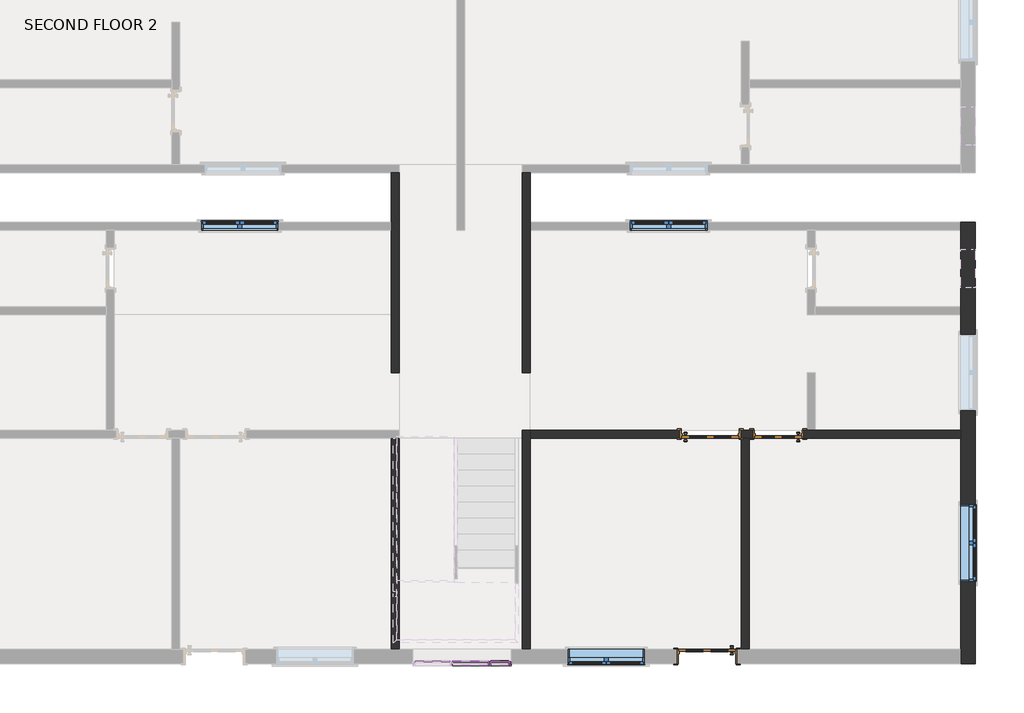
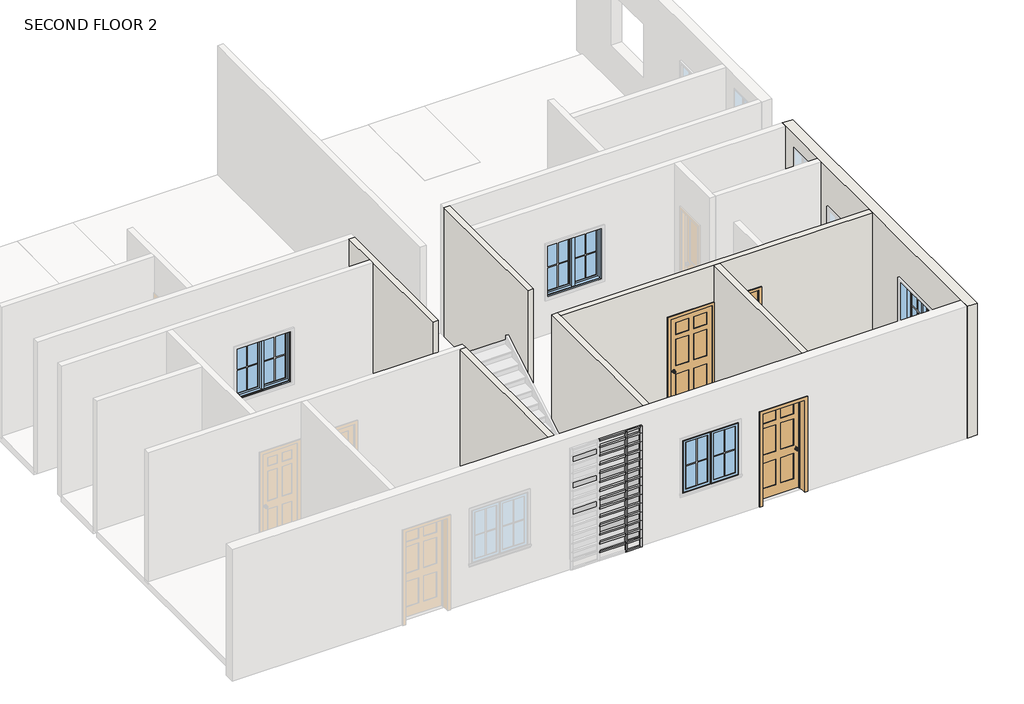
# One storey, part 2 of 4: 57 members, 21 plates, 7 walls, 4 windows, 3 doors.
"""IFC4 building model written with IfcOpenShell, lengths in millimetres."""

from ifc_helpers import new_model, si_unit, frame, origin, place, context, project, spatial, polyline, outline, extrude, faceted_brep, transform, mapped, element, save
from components import door_d66ee888, door_c610b25b, door_c5239341, member_56b223d9, member_a59c64b1, member_06854975, member_b8e7570c, member_a67f877f, member_00eacae2, member_ff422208, member_dc11c383, system_panel_glazed_b3845325, system_panel_glazed_23b8b45c, system_panel_glazed_58d257f9, system_panel_glazed_e426d894, system_panel_glazed_822b3193, window_9200f5ac, window_c2c97eee

model = new_model("IFC4")

# Units and contexts
model_context = context("Model", 3, world=origin())
ifc_project = project(units=[si_unit("LENGTHUNIT", "METRE", prefix="MILLI")], contexts=[model_context])

# Site, building, storey
site = spatial("IfcSite", under=ifc_project)
building = spatial("IfcBuilding", under=site)
storey = spatial("IfcBuildingStorey", under=building, Name="SECOND FLOOR 2", Elevation=6343.9725604)

# Doors
placement = place(None, origin())
door_shape = door_d66ee888(model_context)
element("IfcDoor", 1, ObjectType="Door-Interior-Single-6_Panel-Wood : 30\" x 84\"", at=placement, inside=storey, context=model_context, shape_type="MappedRepresentation", body=[
    mapped(door_shape, transform((777.5862669, -4180.7343836, 6343.9725604), x_axis=(-1.0, 0.0, 0.0), y_axis=(0.0, -1.0, 0.0), z_axis=(0.0, 0.0, 1.0))),
])
door_2_shape = door_c610b25b(model_context)
element("IfcDoor", 2, ObjectType="Door-Interior-Single-6_Panel-Wood : 36\" x 84\"", at=placement, inside=storey, context=model_context, shape_type="MappedRepresentation", body=[
    mapped(door_2_shape, transform((-301.9137331, -4180.7343836, 6343.9725604), x_axis=(1.0, 0.0, 0.0), y_axis=(0.0, 1.0, 0.0), z_axis=(0.0, 0.0, 1.0))),
])
door_3_shape = door_c5239341(model_context)
element("IfcDoor", 3, ObjectType="Door-Interior-Single-6_Panel-Wood : 36\" x 84\"", at=placement, inside=storey, context=model_context, shape_type="MappedRepresentation", body=[
    mapped(door_3_shape, transform((-352.7137331, -7704.9843836, 6343.9725604), x_axis=(-1.0, 0.0, 0.0), y_axis=(0.0, -1.0, 0.0), z_axis=(0.0, 0.0, 1.0))),
])

# Members
member_shape = member_56b223d9(model_context)
element("IfcMember", 4, ObjectType="Rectangular Mullion : 1.5\" x 2.5\" rectangular", at=placement, inside=storey, context=model_context, shape_type="MappedRepresentation", body=[
    mapped(member_shape, transform((-3807.0334597, -7822.4593836, 6343.9725604), x_axis=(1.0, 0.0, 0.0), y_axis=(0.0, -1.0, 0.0), z_axis=(0.0, 0.0, -1.0))),
])
element("IfcMember", 5, ObjectType="Rectangular Mullion : 1.5\" x 2.5\" rectangular", at=placement, inside=storey, context=model_context, shape_type="MappedRepresentation", body=[
    mapped(member_shape, transform((-3807.0334597, -7822.4593836, 6547.1725604), x_axis=(1.0, 0.0, 0.0), y_axis=(0.0, -1.0, 0.0), z_axis=(0.0, 0.0, -1.0))),
])
element("IfcMember", 6, ObjectType="Rectangular Mullion : 1.5\" x 2.5\" rectangular", at=placement, inside=storey, context=model_context, shape_type="MappedRepresentation", body=[
    mapped(member_shape, transform((-3807.0334597, -7822.4593836, 6750.3725604), x_axis=(1.0, 0.0, 0.0), y_axis=(0.0, -1.0, 0.0), z_axis=(0.0, 0.0, -1.0))),
])
element("IfcMember", 7, ObjectType="Rectangular Mullion : 1.5\" x 2.5\" rectangular", at=placement, inside=storey, context=model_context, shape_type="MappedRepresentation", body=[
    mapped(member_shape, transform((-3807.0334597, -7822.4593836, 6953.5725604), x_axis=(1.0, 0.0, 0.0), y_axis=(0.0, -1.0, 0.0), z_axis=(0.0, 0.0, -1.0))),
])
element("IfcMember", 8, ObjectType="Rectangular Mullion : 1.5\" x 2.5\" rectangular", at=placement, inside=storey, context=model_context, shape_type="MappedRepresentation", body=[
    mapped(member_shape, transform((-3807.0334597, -7822.4593836, 7156.7725604), x_axis=(1.0, 0.0, 0.0), y_axis=(0.0, -1.0, 0.0), z_axis=(0.0, 0.0, -1.0))),
])
element("IfcMember", 9, ObjectType="Rectangular Mullion : 1.5\" x 2.5\" rectangular", at=placement, inside=storey, context=model_context, shape_type="MappedRepresentation", body=[
    mapped(member_shape, transform((-3807.0334597, -7822.4593836, 7359.9725604), x_axis=(1.0, 0.0, 0.0), y_axis=(0.0, -1.0, 0.0), z_axis=(0.0, 0.0, -1.0))),
])
element("IfcMember", 10, ObjectType="Rectangular Mullion : 1.5\" x 2.5\" rectangular", at=placement, inside=storey, context=model_context, shape_type="MappedRepresentation", body=[
    mapped(member_shape, transform((-3807.0334597, -7822.4593836, 7563.1725604), x_axis=(1.0, 0.0, 0.0), y_axis=(0.0, -1.0, 0.0), z_axis=(0.0, 0.0, -1.0))),
])
element("IfcMember", 11, ObjectType="Rectangular Mullion : 1.5\" x 2.5\" rectangular", at=placement, inside=storey, context=model_context, shape_type="MappedRepresentation", body=[
    mapped(member_shape, transform((-3807.0334597, -7822.4593836, 7766.3725604), x_axis=(1.0, 0.0, 0.0), y_axis=(0.0, -1.0, 0.0), z_axis=(0.0, 0.0, -1.0))),
])
element("IfcMember", 12, ObjectType="Rectangular Mullion : 1.5\" x 2.5\" rectangular", at=placement, inside=storey, context=model_context, shape_type="MappedRepresentation", body=[
    mapped(member_shape, transform((-3807.0334597, -7822.4593836, 7969.5725604), x_axis=(1.0, 0.0, 0.0), y_axis=(0.0, -1.0, 0.0), z_axis=(0.0, 0.0, -1.0))),
])
element("IfcMember", 13, ObjectType="Rectangular Mullion : 1.5\" x 2.5\" rectangular", at=placement, inside=storey, context=model_context, shape_type="MappedRepresentation", body=[
    mapped(member_shape, transform((-3807.0334597, -7822.4593836, 8172.7725604), x_axis=(1.0, 0.0, 0.0), y_axis=(0.0, -1.0, 0.0), z_axis=(0.0, 0.0, -1.0))),
])
element("IfcMember", 14, ObjectType="Rectangular Mullion : 1.5\" x 2.5\" rectangular", at=placement, inside=storey, context=model_context, shape_type="MappedRepresentation", body=[
    mapped(member_shape, transform((-3807.0334597, -7822.4593836, 8375.9725604), x_axis=(1.0, 0.0, 0.0), y_axis=(0.0, -1.0, 0.0), z_axis=(0.0, 0.0, -1.0))),
])
element("IfcMember", 15, ObjectType="Rectangular Mullion : 1.5\" x 2.5\" rectangular", at=placement, inside=storey, context=model_context, shape_type="MappedRepresentation", body=[
    mapped(member_shape, transform((-3807.0334597, -7822.4593836, 8579.1725604), x_axis=(1.0, 0.0, 0.0), y_axis=(0.0, -1.0, 0.0), z_axis=(0.0, 0.0, -1.0))),
])
element("IfcMember", 16, ObjectType="Rectangular Mullion : 1.5\" x 2.5\" rectangular", at=placement, inside=storey, context=model_context, shape_type="MappedRepresentation", body=[
    mapped(member_shape, transform((-3807.0334597, -7822.4593836, 8782.3725604), x_axis=(1.0, 0.0, 0.0), y_axis=(0.0, -1.0, 0.0), z_axis=(0.0, 0.0, -1.0))),
])
member_2_shape = member_a59c64b1(model_context)
element("IfcMember", 17, ObjectType="Rectangular Mullion : 1.5\" x 2.5\" rectangular", at=placement, inside=storey, context=model_context, shape_type="MappedRepresentation", body=[
    mapped(member_2_shape, transform((-3807.0334597, -7822.4593836, 8985.5725604), x_axis=(1.0, 0.0, 0.0), y_axis=(0.0, -1.0, 0.0), z_axis=(0.0, 0.0, -1.0))),
])
member_3_shape = member_06854975(model_context)
element("IfcMember", 18, ObjectType="Rectangular Mullion : 1.5\" x 2.5\" rectangular", at=placement, inside=storey, context=model_context, shape_type="MappedRepresentation", body=[
    mapped(member_3_shape, transform((-3499.7513929, -7822.4593836, 9151.3551755), x_axis=(0.0, 0.0, 1.0), y_axis=(0.0, -1.0, 0.0), z_axis=(1.0, 0.0, 0.0))),
])
member_4_shape = member_b8e7570c(model_context)
element("IfcMember", 19, ObjectType="Rectangular Mullion : 1.5\" x 2.5\" rectangular", at=placement, inside=storey, context=model_context, shape_type="MappedRepresentation", body=[
    mapped(member_4_shape, transform((-3826.0834597, -7822.4593836, 6547.1725604), x_axis=(0.0, 0.0, 1.0), y_axis=(0.0, -1.0, 0.0), z_axis=(1.0, 0.0, 0.0))),
])
element("IfcMember", 20, ObjectType="Rectangular Mullion : 1.5\" x 2.5\" rectangular", at=placement, inside=storey, context=model_context, shape_type="MappedRepresentation", body=[
    mapped(member_4_shape, transform((-3826.0834597, -7822.4593836, 6750.3725604), x_axis=(0.0, 0.0, 1.0), y_axis=(0.0, -1.0, 0.0), z_axis=(1.0, 0.0, 0.0))),
])
element("IfcMember", 21, ObjectType="Rectangular Mullion : 1.5\" x 2.5\" rectangular", at=placement, inside=storey, context=model_context, shape_type="MappedRepresentation", body=[
    mapped(member_4_shape, transform((-3826.0834597, -7822.4593836, 6953.5725604), x_axis=(0.0, 0.0, 1.0), y_axis=(0.0, -1.0, 0.0), z_axis=(1.0, 0.0, 0.0))),
])
element("IfcMember", 22, ObjectType="Rectangular Mullion : 1.5\" x 2.5\" rectangular", at=placement, inside=storey, context=model_context, shape_type="MappedRepresentation", body=[
    mapped(member_4_shape, transform((-3826.0834597, -7822.4593836, 7156.7725604), x_axis=(0.0, 0.0, 1.0), y_axis=(0.0, -1.0, 0.0), z_axis=(1.0, 0.0, 0.0))),
])
element("IfcMember", 23, ObjectType="Rectangular Mullion : 1.5\" x 2.5\" rectangular", at=placement, inside=storey, context=model_context, shape_type="MappedRepresentation", body=[
    mapped(member_4_shape, transform((-3826.0834597, -7822.4593836, 7359.9725604), x_axis=(0.0, 0.0, 1.0), y_axis=(0.0, -1.0, 0.0), z_axis=(1.0, 0.0, 0.0))),
])
element("IfcMember", 24, ObjectType="Rectangular Mullion : 1.5\" x 2.5\" rectangular", at=placement, inside=storey, context=model_context, shape_type="MappedRepresentation", body=[
    mapped(member_4_shape, transform((-3826.0834597, -7822.4593836, 7563.1725604), x_axis=(0.0, 0.0, 1.0), y_axis=(0.0, -1.0, 0.0), z_axis=(1.0, 0.0, 0.0))),
])
element("IfcMember", 25, ObjectType="Rectangular Mullion : 1.5\" x 2.5\" rectangular", at=placement, inside=storey, context=model_context, shape_type="MappedRepresentation", body=[
    mapped(member_4_shape, transform((-3826.0834597, -7822.4593836, 7766.3725604), x_axis=(0.0, 0.0, 1.0), y_axis=(0.0, -1.0, 0.0), z_axis=(1.0, 0.0, 0.0))),
])
element("IfcMember", 26, ObjectType="Rectangular Mullion : 1.5\" x 2.5\" rectangular", at=placement, inside=storey, context=model_context, shape_type="MappedRepresentation", body=[
    mapped(member_4_shape, transform((-3826.0834597, -7822.4593836, 7969.5725604), x_axis=(0.0, 0.0, 1.0), y_axis=(0.0, -1.0, 0.0), z_axis=(1.0, 0.0, 0.0))),
])
element("IfcMember", 27, ObjectType="Rectangular Mullion : 1.5\" x 2.5\" rectangular", at=placement, inside=storey, context=model_context, shape_type="MappedRepresentation", body=[
    mapped(member_4_shape, transform((-3826.0834597, -7822.4593836, 8172.7725604), x_axis=(0.0, 0.0, 1.0), y_axis=(0.0, -1.0, 0.0), z_axis=(1.0, 0.0, 0.0))),
])
element("IfcMember", 28, ObjectType="Rectangular Mullion : 1.5\" x 2.5\" rectangular", at=placement, inside=storey, context=model_context, shape_type="MappedRepresentation", body=[
    mapped(member_4_shape, transform((-3826.0834597, -7822.4593836, 8375.9725604), x_axis=(0.0, 0.0, 1.0), y_axis=(0.0, -1.0, 0.0), z_axis=(1.0, 0.0, 0.0))),
])
element("IfcMember", 29, ObjectType="Rectangular Mullion : 1.5\" x 2.5\" rectangular", at=placement, inside=storey, context=model_context, shape_type="MappedRepresentation", body=[
    mapped(member_4_shape, transform((-3826.0834597, -7822.4593836, 8579.1725604), x_axis=(0.0, 0.0, 1.0), y_axis=(0.0, -1.0, 0.0), z_axis=(1.0, 0.0, 0.0))),
])
element("IfcMember", 30, ObjectType="Rectangular Mullion : 1.5\" x 2.5\" rectangular", at=placement, inside=storey, context=model_context, shape_type="MappedRepresentation", body=[
    mapped(member_4_shape, transform((-3826.0834597, -7822.4593836, 8782.3725604), x_axis=(0.0, 0.0, 1.0), y_axis=(0.0, -1.0, 0.0), z_axis=(1.0, 0.0, 0.0))),
])
element("IfcMember", 31, ObjectType="Rectangular Mullion : 1.5\" x 2.5\" rectangular", at=placement, inside=storey, context=model_context, shape_type="MappedRepresentation", body=[
    mapped(member_4_shape, transform((-3826.0834597, -7822.4593836, 8985.5725604), x_axis=(0.0, 0.0, 1.0), y_axis=(0.0, -1.0, 0.0), z_axis=(1.0, 0.0, 0.0))),
])
member_5_shape = member_a67f877f(model_context)
element("IfcMember", 32, ObjectType="Rectangular Mullion : 1.5\" x 2.5\" rectangular", at=placement, inside=storey, context=model_context, shape_type="MappedRepresentation", body=[
    mapped(member_5_shape, transform((-3826.0834597, -7822.4593836, 9151.3551755), x_axis=(0.0, 0.0, 1.0), y_axis=(0.0, -1.0, 0.0), z_axis=(1.0, 0.0, 0.0))),
])
element("IfcMember", 33, ObjectType="Rectangular Mullion : 1.5\" x 2.5\" rectangular", at=placement, inside=storey, context=model_context, shape_type="MappedRepresentation", body=[
    mapped(member_3_shape, transform((-3787.9834597, -7822.4593836, 6343.9725604), x_axis=(0.0, 0.0, -1.0), y_axis=(0.0, -1.0, 0.0), z_axis=(-1.0, 0.0, 0.0))),
])
member_6_shape = member_00eacae2(model_context)
element("IfcMember", 34, ObjectType="Rectangular Mullion : 1.5\" x 2.5\" rectangular", at=placement, inside=storey, context=model_context, shape_type="MappedRepresentation", body=[
    mapped(member_6_shape, transform((-3499.7513929, -7822.4593836, 6547.1725604), x_axis=(0.0, 0.0, 1.0), y_axis=(0.0, -1.0, 0.0), z_axis=(1.0, 0.0, 0.0))),
])
element("IfcMember", 35, ObjectType="Rectangular Mullion : 1.5\" x 2.5\" rectangular", at=placement, inside=storey, context=model_context, shape_type="MappedRepresentation", body=[
    mapped(member_6_shape, transform((-3499.7513929, -7822.4593836, 6750.3725604), x_axis=(0.0, 0.0, 1.0), y_axis=(0.0, -1.0, 0.0), z_axis=(1.0, 0.0, 0.0))),
])
element("IfcMember", 36, ObjectType="Rectangular Mullion : 1.5\" x 2.5\" rectangular", at=placement, inside=storey, context=model_context, shape_type="MappedRepresentation", body=[
    mapped(member_6_shape, transform((-3499.7513929, -7822.4593836, 6953.5725604), x_axis=(0.0, 0.0, 1.0), y_axis=(0.0, -1.0, 0.0), z_axis=(1.0, 0.0, 0.0))),
])
element("IfcMember", 37, ObjectType="Rectangular Mullion : 1.5\" x 2.5\" rectangular", at=placement, inside=storey, context=model_context, shape_type="MappedRepresentation", body=[
    mapped(member_6_shape, transform((-3499.7513929, -7822.4593836, 7156.7725604), x_axis=(0.0, 0.0, 1.0), y_axis=(0.0, -1.0, 0.0), z_axis=(1.0, 0.0, 0.0))),
])
element("IfcMember", 38, ObjectType="Rectangular Mullion : 1.5\" x 2.5\" rectangular", at=placement, inside=storey, context=model_context, shape_type="MappedRepresentation", body=[
    mapped(member_6_shape, transform((-3499.7513929, -7822.4593836, 7359.9725604), x_axis=(0.0, 0.0, 1.0), y_axis=(0.0, -1.0, 0.0), z_axis=(1.0, 0.0, 0.0))),
])
element("IfcMember", 39, ObjectType="Rectangular Mullion : 1.5\" x 2.5\" rectangular", at=placement, inside=storey, context=model_context, shape_type="MappedRepresentation", body=[
    mapped(member_6_shape, transform((-3499.7513929, -7822.4593836, 7563.1725604), x_axis=(0.0, 0.0, 1.0), y_axis=(0.0, -1.0, 0.0), z_axis=(1.0, 0.0, 0.0))),
])
element("IfcMember", 40, ObjectType="Rectangular Mullion : 1.5\" x 2.5\" rectangular", at=placement, inside=storey, context=model_context, shape_type="MappedRepresentation", body=[
    mapped(member_6_shape, transform((-3499.7513929, -7822.4593836, 7766.3725604), x_axis=(0.0, 0.0, 1.0), y_axis=(0.0, -1.0, 0.0), z_axis=(1.0, 0.0, 0.0))),
])
element("IfcMember", 41, ObjectType="Rectangular Mullion : 1.5\" x 2.5\" rectangular", at=placement, inside=storey, context=model_context, shape_type="MappedRepresentation", body=[
    mapped(member_6_shape, transform((-3499.7513929, -7822.4593836, 7969.5725604), x_axis=(0.0, 0.0, 1.0), y_axis=(0.0, -1.0, 0.0), z_axis=(1.0, 0.0, 0.0))),
])
element("IfcMember", 42, ObjectType="Rectangular Mullion : 1.5\" x 2.5\" rectangular", at=placement, inside=storey, context=model_context, shape_type="MappedRepresentation", body=[
    mapped(member_6_shape, transform((-3499.7513929, -7822.4593836, 8172.7725604), x_axis=(0.0, 0.0, 1.0), y_axis=(0.0, -1.0, 0.0), z_axis=(1.0, 0.0, 0.0))),
])
element("IfcMember", 43, ObjectType="Rectangular Mullion : 1.5\" x 2.5\" rectangular", at=placement, inside=storey, context=model_context, shape_type="MappedRepresentation", body=[
    mapped(member_6_shape, transform((-3499.7513929, -7822.4593836, 8375.9725604), x_axis=(0.0, 0.0, 1.0), y_axis=(0.0, -1.0, 0.0), z_axis=(1.0, 0.0, 0.0))),
])
element("IfcMember", 44, ObjectType="Rectangular Mullion : 1.5\" x 2.5\" rectangular", at=placement, inside=storey, context=model_context, shape_type="MappedRepresentation", body=[
    mapped(member_6_shape, transform((-3499.7513929, -7822.4593836, 8579.1725604), x_axis=(0.0, 0.0, 1.0), y_axis=(0.0, -1.0, 0.0), z_axis=(1.0, 0.0, 0.0))),
])
element("IfcMember", 45, ObjectType="Rectangular Mullion : 1.5\" x 2.5\" rectangular", at=placement, inside=storey, context=model_context, shape_type="MappedRepresentation", body=[
    mapped(member_6_shape, transform((-3499.7513929, -7822.4593836, 8782.3725604), x_axis=(0.0, 0.0, 1.0), y_axis=(0.0, -1.0, 0.0), z_axis=(1.0, 0.0, 0.0))),
])
element("IfcMember", 46, ObjectType="Rectangular Mullion : 1.5\" x 2.5\" rectangular", at=placement, inside=storey, context=model_context, shape_type="MappedRepresentation", body=[
    mapped(member_6_shape, transform((-3499.7513929, -7822.4593836, 8985.5725604), x_axis=(0.0, 0.0, 1.0), y_axis=(0.0, -1.0, 0.0), z_axis=(1.0, 0.0, 0.0))),
])
member_7_shape = member_ff422208(model_context)
element("IfcMember", 47, ObjectType="Rectangular Mullion : 1.5\" x 2.5\" rectangular", at=placement, inside=storey, context=model_context, shape_type="MappedRepresentation", body=[
    mapped(member_7_shape, transform((-3461.6513929, -7822.4593836, 6343.9725604), x_axis=(1.0, 0.0, 0.0), y_axis=(0.0, -1.0, 0.0), z_axis=(0.0, 0.0, -1.0))),
])
element("IfcMember", 48, ObjectType="Rectangular Mullion : 1.5\" x 2.5\" rectangular", at=placement, inside=storey, context=model_context, shape_type="MappedRepresentation", body=[
    mapped(member_7_shape, transform((-3461.6513929, -7822.4593836, 6547.1725604), x_axis=(1.0, 0.0, 0.0), y_axis=(0.0, -1.0, 0.0), z_axis=(0.0, 0.0, -1.0))),
])
element("IfcMember", 49, ObjectType="Rectangular Mullion : 1.5\" x 2.5\" rectangular", at=placement, inside=storey, context=model_context, shape_type="MappedRepresentation", body=[
    mapped(member_7_shape, transform((-3461.6513929, -7822.4593836, 6750.3725604), x_axis=(1.0, 0.0, 0.0), y_axis=(0.0, -1.0, 0.0), z_axis=(0.0, 0.0, -1.0))),
])
element("IfcMember", 50, ObjectType="Rectangular Mullion : 1.5\" x 2.5\" rectangular", at=placement, inside=storey, context=model_context, shape_type="MappedRepresentation", body=[
    mapped(member_7_shape, transform((-3461.6513929, -7822.4593836, 6953.5725604), x_axis=(1.0, 0.0, 0.0), y_axis=(0.0, -1.0, 0.0), z_axis=(0.0, 0.0, -1.0))),
])
element("IfcMember", 51, ObjectType="Rectangular Mullion : 1.5\" x 2.5\" rectangular", at=placement, inside=storey, context=model_context, shape_type="MappedRepresentation", body=[
    mapped(member_7_shape, transform((-3461.6513929, -7822.4593836, 7156.7725604), x_axis=(1.0, 0.0, 0.0), y_axis=(0.0, -1.0, 0.0), z_axis=(0.0, 0.0, -1.0))),
])
element("IfcMember", 52, ObjectType="Rectangular Mullion : 1.5\" x 2.5\" rectangular", at=placement, inside=storey, context=model_context, shape_type="MappedRepresentation", body=[
    mapped(member_7_shape, transform((-3461.6513929, -7822.4593836, 7359.9725604), x_axis=(1.0, 0.0, 0.0), y_axis=(0.0, -1.0, 0.0), z_axis=(0.0, 0.0, -1.0))),
])
element("IfcMember", 53, ObjectType="Rectangular Mullion : 1.5\" x 2.5\" rectangular", at=placement, inside=storey, context=model_context, shape_type="MappedRepresentation", body=[
    mapped(member_7_shape, transform((-3461.6513929, -7822.4593836, 7563.1725604), x_axis=(1.0, 0.0, 0.0), y_axis=(0.0, -1.0, 0.0), z_axis=(0.0, 0.0, -1.0))),
])
element("IfcMember", 54, ObjectType="Rectangular Mullion : 1.5\" x 2.5\" rectangular", at=placement, inside=storey, context=model_context, shape_type="MappedRepresentation", body=[
    mapped(member_7_shape, transform((-3461.6513929, -7822.4593836, 7766.3725604), x_axis=(1.0, 0.0, 0.0), y_axis=(0.0, -1.0, 0.0), z_axis=(0.0, 0.0, -1.0))),
])
element("IfcMember", 55, ObjectType="Rectangular Mullion : 1.5\" x 2.5\" rectangular", at=placement, inside=storey, context=model_context, shape_type="MappedRepresentation", body=[
    mapped(member_7_shape, transform((-3461.6513929, -7822.4593836, 7969.5725604), x_axis=(1.0, 0.0, 0.0), y_axis=(0.0, -1.0, 0.0), z_axis=(0.0, 0.0, -1.0))),
])
element("IfcMember", 56, ObjectType="Rectangular Mullion : 1.5\" x 2.5\" rectangular", at=placement, inside=storey, context=model_context, shape_type="MappedRepresentation", body=[
    mapped(member_7_shape, transform((-3461.6513929, -7822.4593836, 8172.7725604), x_axis=(1.0, 0.0, 0.0), y_axis=(0.0, -1.0, 0.0), z_axis=(0.0, 0.0, -1.0))),
])
element("IfcMember", 57, ObjectType="Rectangular Mullion : 1.5\" x 2.5\" rectangular", at=placement, inside=storey, context=model_context, shape_type="MappedRepresentation", body=[
    mapped(member_7_shape, transform((-3461.6513929, -7822.4593836, 8375.9725604), x_axis=(1.0, 0.0, 0.0), y_axis=(0.0, -1.0, 0.0), z_axis=(0.0, 0.0, -1.0))),
])
element("IfcMember", 58, ObjectType="Rectangular Mullion : 1.5\" x 2.5\" rectangular", at=placement, inside=storey, context=model_context, shape_type="MappedRepresentation", body=[
    mapped(member_7_shape, transform((-3461.6513929, -7822.4593836, 8579.1725604), x_axis=(1.0, 0.0, 0.0), y_axis=(0.0, -1.0, 0.0), z_axis=(0.0, 0.0, -1.0))),
])
element("IfcMember", 59, ObjectType="Rectangular Mullion : 1.5\" x 2.5\" rectangular", at=placement, inside=storey, context=model_context, shape_type="MappedRepresentation", body=[
    mapped(member_7_shape, transform((-3461.6513929, -7822.4593836, 8782.3725604), x_axis=(1.0, 0.0, 0.0), y_axis=(0.0, -1.0, 0.0), z_axis=(0.0, 0.0, -1.0))),
])
member_8_shape = member_dc11c383(model_context)
element("IfcMember", 60, ObjectType="Rectangular Mullion : 1.5\" x 2.5\" rectangular", at=placement, inside=storey, context=model_context, shape_type="MappedRepresentation", body=[
    mapped(member_8_shape, transform((-3461.6513929, -7822.4593836, 8985.5725604), x_axis=(1.0, 0.0, 0.0), y_axis=(0.0, -1.0, 0.0), z_axis=(0.0, 0.0, -1.0))),
])

# Plates
system_panel_glazed_shape = system_panel_glazed_b3845325(model_context)
element("IfcPlate", 61, ObjectType="System Panel : Glazed", at=placement, inside=storey, context=model_context, shape_type="MappedRepresentation", body=[
    mapped(system_panel_glazed_shape, transform((-4711.9084599, -7822.4593836, 7582.2225604), x_axis=(1.0, 0.0, 0.0), y_axis=(0.0, 1.0, 0.0), z_axis=(0.0, 0.0, 1.0))),
])
element("IfcPlate", 62, ObjectType="System Panel : Glazed", at=placement, inside=storey, context=model_context, shape_type="MappedRepresentation", body=[
    mapped(system_panel_glazed_shape, transform((-4711.9084599, -7822.4593836, 8191.8225604), x_axis=(1.0, 0.0, 0.0), y_axis=(0.0, 1.0, 0.0), z_axis=(0.0, 0.0, 1.0))),
])
element("IfcPlate", 63, ObjectType="System Panel : Glazed", at=placement, inside=storey, context=model_context, shape_type="MappedRepresentation", body=[
    mapped(system_panel_glazed_shape, transform((-4711.9084599, -7822.4593836, 8801.4225604), x_axis=(1.0, 0.0, 0.0), y_axis=(0.0, 1.0, 0.0), z_axis=(0.0, 0.0, 1.0))),
])
system_panel_glazed_2_shape = system_panel_glazed_23b8b45c(model_context)
element("IfcPlate", 64, ObjectType="System Panel : Glazed", at=placement, inside=storey, context=model_context, shape_type="MappedRepresentation", body=[
    mapped(system_panel_glazed_2_shape, transform((-4111.8334597, -7822.4593836, 6972.6225604), x_axis=(1.0, 0.0, 0.0), y_axis=(0.0, 1.0, 0.0), z_axis=(0.0, 0.0, 1.0))),
])
element("IfcPlate", 65, ObjectType="System Panel : Glazed", at=placement, inside=storey, context=model_context, shape_type="MappedRepresentation", body=[
    mapped(system_panel_glazed_2_shape, transform((-4111.8334597, -7822.4593836, 7582.2225604), x_axis=(1.0, 0.0, 0.0), y_axis=(0.0, 1.0, 0.0), z_axis=(0.0, 0.0, 1.0))),
])
element("IfcPlate", 66, ObjectType="System Panel : Glazed", at=placement, inside=storey, context=model_context, shape_type="MappedRepresentation", body=[
    mapped(system_panel_glazed_2_shape, transform((-4111.8334597, -7822.4593836, 8191.8225604), x_axis=(1.0, 0.0, 0.0), y_axis=(0.0, 1.0, 0.0), z_axis=(0.0, 0.0, 1.0))),
])
element("IfcPlate", 67, ObjectType="System Panel : Glazed", at=placement, inside=storey, context=model_context, shape_type="MappedRepresentation", body=[
    mapped(system_panel_glazed_2_shape, transform((-4111.8334597, -7822.4593836, 8801.4225604), x_axis=(1.0, 0.0, 0.0), y_axis=(0.0, 1.0, 0.0), z_axis=(0.0, 0.0, 1.0))),
])
system_panel_glazed_3_shape = system_panel_glazed_58d257f9(model_context)
element("IfcPlate", 68, ObjectType="System Panel : Glazed", at=placement, inside=storey, context=model_context, shape_type="MappedRepresentation", body=[
    mapped(system_panel_glazed_3_shape, transform((-3643.8674263, -7822.4593836, 6382.0725604), x_axis=(1.0, 0.0, 0.0), y_axis=(0.0, 1.0, 0.0), z_axis=(0.0, 0.0, 1.0))),
])
system_panel_glazed_4_shape = system_panel_glazed_e426d894(model_context)
element("IfcPlate", 69, ObjectType="System Panel : Glazed", at=placement, inside=storey, context=model_context, shape_type="MappedRepresentation", body=[
    mapped(system_panel_glazed_4_shape, transform((-3643.8674263, -7822.4593836, 6566.2225604), x_axis=(1.0, 0.0, 0.0), y_axis=(0.0, 1.0, 0.0), z_axis=(0.0, 0.0, 1.0))),
])
element("IfcPlate", 70, ObjectType="System Panel : Glazed", at=placement, inside=storey, context=model_context, shape_type="MappedRepresentation", body=[
    mapped(system_panel_glazed_4_shape, transform((-3643.8674263, -7822.4593836, 6769.4225604), x_axis=(1.0, 0.0, 0.0), y_axis=(0.0, 1.0, 0.0), z_axis=(0.0, 0.0, 1.0))),
])
element("IfcPlate", 71, ObjectType="System Panel : Glazed", at=placement, inside=storey, context=model_context, shape_type="MappedRepresentation", body=[
    mapped(system_panel_glazed_4_shape, transform((-3643.8674263, -7822.4593836, 7175.8225604), x_axis=(1.0, 0.0, 0.0), y_axis=(0.0, 1.0, 0.0), z_axis=(0.0, 0.0, 1.0))),
])
element("IfcPlate", 72, ObjectType="System Panel : Glazed", at=placement, inside=storey, context=model_context, shape_type="MappedRepresentation", body=[
    mapped(system_panel_glazed_4_shape, transform((-3643.8674263, -7822.4593836, 7379.0225604), x_axis=(1.0, 0.0, 0.0), y_axis=(0.0, 1.0, 0.0), z_axis=(0.0, 0.0, 1.0))),
])
element("IfcPlate", 73, ObjectType="System Panel : Glazed", at=placement, inside=storey, context=model_context, shape_type="MappedRepresentation", body=[
    mapped(system_panel_glazed_4_shape, transform((-3643.8674263, -7822.4593836, 7785.4225604), x_axis=(1.0, 0.0, 0.0), y_axis=(0.0, 1.0, 0.0), z_axis=(0.0, 0.0, 1.0))),
])
element("IfcPlate", 74, ObjectType="System Panel : Glazed", at=placement, inside=storey, context=model_context, shape_type="MappedRepresentation", body=[
    mapped(system_panel_glazed_4_shape, transform((-3643.8674263, -7822.4593836, 7988.6225604), x_axis=(1.0, 0.0, 0.0), y_axis=(0.0, 1.0, 0.0), z_axis=(0.0, 0.0, 1.0))),
])
element("IfcPlate", 75, ObjectType="System Panel : Glazed", at=placement, inside=storey, context=model_context, shape_type="MappedRepresentation", body=[
    mapped(system_panel_glazed_4_shape, transform((-3643.8674263, -7822.4593836, 8395.0225604), x_axis=(1.0, 0.0, 0.0), y_axis=(0.0, 1.0, 0.0), z_axis=(0.0, 0.0, 1.0))),
])
element("IfcPlate", 76, ObjectType="System Panel : Glazed", at=placement, inside=storey, context=model_context, shape_type="MappedRepresentation", body=[
    mapped(system_panel_glazed_4_shape, transform((-3643.8674263, -7822.4593836, 8598.2225604), x_axis=(1.0, 0.0, 0.0), y_axis=(0.0, 1.0, 0.0), z_axis=(0.0, 0.0, 1.0))),
])
element("IfcPlate", 77, ObjectType="System Panel : Glazed", at=placement, inside=storey, context=model_context, shape_type="MappedRepresentation", body=[
    mapped(system_panel_glazed_4_shape, transform((-3643.8674263, -7822.4593836, 6972.6225604), x_axis=(1.0, 0.0, 0.0), y_axis=(0.0, 1.0, 0.0), z_axis=(0.0, 0.0, 1.0))),
])
element("IfcPlate", 78, ObjectType="System Panel : Glazed", at=placement, inside=storey, context=model_context, shape_type="MappedRepresentation", body=[
    mapped(system_panel_glazed_4_shape, transform((-3643.8674263, -7822.4593836, 7582.2225604), x_axis=(1.0, 0.0, 0.0), y_axis=(0.0, 1.0, 0.0), z_axis=(0.0, 0.0, 1.0))),
])
element("IfcPlate", 79, ObjectType="System Panel : Glazed", at=placement, inside=storey, context=model_context, shape_type="MappedRepresentation", body=[
    mapped(system_panel_glazed_4_shape, transform((-3643.8674263, -7822.4593836, 8191.8225604), x_axis=(1.0, 0.0, 0.0), y_axis=(0.0, 1.0, 0.0), z_axis=(0.0, 0.0, 1.0))),
])
element("IfcPlate", 80, ObjectType="System Panel : Glazed", at=placement, inside=storey, context=model_context, shape_type="MappedRepresentation", body=[
    mapped(system_panel_glazed_4_shape, transform((-3643.8674263, -7822.4593836, 8801.4225604), x_axis=(1.0, 0.0, 0.0), y_axis=(0.0, 1.0, 0.0), z_axis=(0.0, 0.0, 1.0))),
])
system_panel_glazed_5_shape = system_panel_glazed_822b3193(model_context)
element("IfcPlate", 81, ObjectType="System Panel : Glazed", at=placement, inside=storey, context=model_context, shape_type="MappedRepresentation", body=[
    mapped(system_panel_glazed_5_shape, transform((-3643.8674263, -7822.4593836, 9004.6225604), x_axis=(1.0, 0.0, 0.0), y_axis=(0.0, 1.0, 0.0), z_axis=(0.0, 0.0, 1.0))),
])

# Walls
element("IfcWall", 82, ObjectType="Inner Wall 5\"", at=placement, inside=storey, context=model_context, shape_type="Brep", body=[
    faceted_brep([(-5369.2137331, -24.6593836, 6343.9725604), (-5369.2137331, -812.0593836, 6343.9725604), (-5369.2137331, -939.0593836, 6343.9725604), (-5369.2137331, -3199.6593836, 6343.9725604), (-5369.2137331, -3199.6593836, 9391.9725604), (-5369.2137331, -939.0593836, 9391.9725604), (-5369.2137331, -812.0593836, 9391.9725604), (-5369.2137331, -24.6593836, 9391.9725604), (-5242.2137331, -24.6593836, 6343.9725604), (-5242.2137331, -24.6593836, 9391.9725604), (-5242.2137331, -3199.6593836, 9391.9725604), (-5242.2137331, -3199.6593836, 6343.9725604)], [[[0, 1, 2, 3, 4, 5, 6, 7]], [[8, 9, 10, 11]], [[3, 2, 1, 0, 8, 11]], [[4, 3, 11, 10]], [[7, 6, 5, 4, 10, 9]], [[0, 7, 9, 8]]]),
])
element("IfcWall", 83, ObjectType="Inner Wall 5\"", at=placement, inside=storey, context=model_context, shape_type="Brep", body=[
    faceted_brep([(-3286.4137331, -24.6593836, 6343.9725604), (-3286.4137331, -3199.6593836, 6343.9725604), (-3286.4137331, -3199.6593836, 9391.9725604), (-3286.4137331, -24.6593836, 9391.9725604), (-3159.4137331, -24.6593836, 6343.9725604), (-3159.4137331, -24.6593836, 9391.9725604), (-3159.4137331, -812.0593836, 9391.9725604), (-3159.4137331, -939.0593836, 9391.9725604), (-3159.4137331, -3199.6593836, 9391.9725604), (-3159.4137331, -3199.6593836, 6343.9725604), (-3159.4137331, -939.0593836, 6343.9725604), (-3159.4137331, -812.0593836, 6343.9725604)], [[[0, 1, 2, 3]], [[4, 5, 6, 7, 8, 9, 10, 11]], [[1, 0, 4, 11, 10, 9]], [[2, 1, 9, 8]], [[3, 2, 8, 7, 6, 5]], [[0, 3, 5, 4]]]),
])
element("IfcWall", 84, ObjectType="Inner Wall 5\"", at=placement, inside=storey, context=model_context, shape_type="SweptSolid", body=[
    extrude(outline(polyline([(-5242.2137331, -4241.0593836), (-5242.2137331, -7593.8593836), (-5369.2137331, -7593.8593836), (-5369.2137331, -4241.0593836), (-5242.2137331, -4241.0593836)])), frame((0.0, 0.0, 6343.9725604), z_axis=(0.0, 0.0, 1.0), x_axis=(1.0, 0.0, 0.0)), (0.0, 0.0, 1.0), 3048.0),
])
element("IfcWall", 85, ObjectType="Inner Wall 5\"", at=placement, inside=storey, context=model_context, shape_type="Brep", body=[
    faceted_brep([(-3159.4137331, -7593.8593836, 6343.9725604), (-3159.4137331, -4241.0593836, 6343.9725604), (-3159.4137331, -4114.0593836, 6343.9725604), (-3159.4137331, -4114.0593836, 9391.9725604), (-3159.4137331, -4241.0593836, 9391.9725604), (-3159.4137331, -7593.8593836, 9391.9725604), (-3286.4137331, -7593.8593836, 6343.9725604), (-3286.4137331, -7593.8593836, 9391.9725604), (-3286.4137331, -4114.0593836, 9391.9725604), (-3286.4137331, -4114.0593836, 6343.9725604)], [[[0, 1, 2, 3, 4, 5]], [[6, 7, 8, 9]], [[2, 1, 0, 6, 9]], [[5, 4, 3, 8, 7]], [[0, 5, 7, 6]], [[3, 2, 9, 8]]]),
])
element("IfcWall", 86, ObjectType="Inner Wall 5\"", at=placement, inside=storey, context=model_context, shape_type="Brep", body=[
    faceted_brep([(3673.1862669, -4241.0593836, 9391.9725604), (320.3862669, -4241.0593836, 9391.9725604), (193.3862669, -4241.0593836, 9391.9725604), (-3159.4137331, -4241.0593836, 9391.9725604), (-3159.4137331, -4241.0593836, 6343.9725604), (-784.5137331, -4241.0593836, 6343.9725604), (-784.5137331, -4241.0593836, 8502.9725604), (180.6862669, -4241.0593836, 8502.9725604), (180.6862669, -4241.0593836, 6343.9725604), (193.3862669, -4241.0593836, 6343.9725604), (320.3862669, -4241.0593836, 6343.9725604), (371.1862669, -4241.0593836, 6343.9725604), (371.1862669, -4241.0593836, 8502.9725604), (1183.9862669, -4241.0593836, 8502.9725604), (1183.9862669, -4241.0593836, 6343.9725604), (3673.1862669, -4241.0593836, 6343.9725604), (-3159.4137331, -4114.0593836, 9391.9725604), (1234.7862669, -4114.0593836, 9391.9725604), (1361.7862669, -4114.0593836, 9391.9725604), (3673.1862669, -4114.0593836, 9391.9725604), (3673.1862669, -4114.0593836, 6343.9725604), (1361.7862669, -4114.0593836, 6343.9725604), (1234.7862669, -4114.0593836, 6343.9725604), (1183.9862669, -4114.0593836, 6343.9725604), (1183.9862669, -4114.0593836, 8502.9725604), (371.1862669, -4114.0593836, 8502.9725604), (371.1862669, -4114.0593836, 6343.9725604), (180.6862669, -4114.0593836, 6343.9725604), (180.6862669, -4114.0593836, 8502.9725604), (-784.5137331, -4114.0593836, 8502.9725604), (-784.5137331, -4114.0593836, 6343.9725604), (-3159.4137331, -4114.0593836, 6343.9725604)], [[[0, 1, 2, 3, 4, 5, 6, 7, 8, 9, 10, 11, 12, 13, 14, 15]], [[16, 17, 18, 19, 20, 21, 22, 23, 24, 25, 26, 27, 28, 29, 30, 31]], [[4, 31, 30, 5]], [[20, 15, 14, 23, 22, 21]], [[8, 27, 26, 11, 10, 9]], [[3, 2, 1, 0, 19, 18, 17, 16]], [[4, 3, 16, 31]], [[0, 15, 20, 19]], [[7, 28, 27, 8]], [[28, 7, 6, 29]], [[29, 6, 5, 30]], [[25, 12, 11, 26]], [[12, 25, 24, 13]], [[13, 24, 23, 14]]]),
])
element("IfcWall", 87, ObjectType="Inner Wall 5\"", at=placement, inside=storey, context=model_context, shape_type="SweptSolid", body=[
    extrude(outline(polyline([(320.3862669, -4241.0593836), (320.3862669, -7593.8593836), (193.3862669, -7593.8593836), (193.3862669, -4241.0593836), (320.3862669, -4241.0593836)])), frame((0.0, 0.0, 6343.9725604), z_axis=(0.0, 0.0, 1.0), x_axis=(1.0, 0.0, 0.0)), (0.0, 0.0, 1.0), 3048.0),
])
element("IfcWall", 88, ObjectType="outer wall 9\"", at=placement, inside=storey, context=model_context, shape_type="Brep", body=[
    faceted_brep([(3901.7862669, -7822.4593836, 6343.9725604), (3901.7862669, -812.0593836, 6343.9725604), (3901.7862669, -812.0593836, 9391.9725604), (3901.7862669, -7822.4593836, 9391.9725604), (3901.7862669, -3809.2593836, 8477.5725604), (3901.7862669, -2590.0593836, 8477.5725604), (3901.7862669, -2590.0593836, 7258.3725604), (3901.7862669, -3809.2593836, 7258.3725604), (3901.7862669, -6514.3593836, 8477.5725604), (3901.7862669, -5295.1593836, 8477.5725604), (3901.7862669, -5295.1593836, 7258.3725604), (3901.7862669, -6514.3593836, 7258.3725604), (3901.7862669, -1853.4593836, 9087.1725604), (3901.7862669, -1243.8593836, 9087.1725604), (3901.7862669, -1243.8593836, 8477.5725604), (3901.7862669, -1853.4593836, 8477.5725604), (3673.1862669, -7822.4593836, 6343.9725604), (3673.1862669, -7822.4593836, 9391.9725604), (3673.1862669, -7593.8593836, 9391.9725604), (3673.1862669, -4241.0593836, 9391.9725604), (3673.1862669, -4114.0593836, 9391.9725604), (3673.1862669, -2285.2593836, 9391.9725604), (3673.1862669, -2158.2593836, 9391.9725604), (3673.1862669, -939.0593836, 9391.9725604), (3673.1862669, -812.0593836, 9391.9725604), (3673.1862669, -812.0593836, 6343.9725604), (3673.1862669, -939.0593836, 6343.9725604), (3673.1862669, -2158.2593836, 6343.9725604), (3673.1862669, -2285.2593836, 6343.9725604), (3673.1862669, -4114.0593836, 6343.9725604), (3673.1862669, -4241.0593836, 6343.9725604), (3673.1862669, -7593.8593836, 6343.9725604), (3673.1862669, -3809.2593836, 8477.5725604), (3673.1862669, -3809.2593836, 7258.3725604), (3673.1862669, -2590.0593836, 7258.3725604), (3673.1862669, -2590.0593836, 8477.5725604), (3673.1862669, -6514.3593836, 8477.5725604), (3673.1862669, -6514.3593836, 7258.3725604), (3673.1862669, -5295.1593836, 7258.3725604), (3673.1862669, -5295.1593836, 8477.5725604), (3673.1862669, -1853.4593836, 9087.1725604), (3673.1862669, -1853.4593836, 8477.5725604), (3673.1862669, -1243.8593836, 8477.5725604), (3673.1862669, -1243.8593836, 9087.1725604)], [[[0, 1, 2, 3], [4, 5, 6, 7], [8, 9, 10, 11], [12, 13, 14, 15]], [[16, 17, 18, 19, 20, 21, 22, 23, 24, 25, 26, 27, 28, 29, 30, 31], [32, 33, 34, 35], [36, 37, 38, 39], [40, 41, 42, 43]], [[1, 0, 16, 31, 30, 29, 28, 27, 26, 25]], [[3, 2, 24, 23, 22, 21, 20, 19, 18, 17]], [[0, 3, 17, 16]], [[2, 1, 25, 24]], [[33, 32, 4, 7]], [[34, 33, 7, 6]], [[35, 34, 6, 5]], [[32, 35, 5, 4]], [[37, 36, 8, 11]], [[38, 37, 11, 10]], [[39, 38, 10, 9]], [[36, 39, 9, 8]], [[41, 40, 12, 15]], [[42, 41, 15, 14]], [[43, 42, 14, 13]], [[40, 43, 13, 12]]]),
])

# Windows
window_shape = window_9200f5ac(model_context)
element("IfcWindow", 89, ObjectType="Window-Casement-Double : 48\" x 48\"", at=placement, inside=storey, context=model_context, shape_type="MappedRepresentation", body=[
    mapped(window_shape, transform((3787.4862669, -5904.7593836, 6343.9725604), x_axis=(0.0, -1.0, 0.0), y_axis=(1.0, 0.0, 0.0), z_axis=(0.0, 0.0, 1.0))),
])
element("IfcWindow", 90, ObjectType="Window-Casement-Double : 48\" x 48\"", at=placement, inside=storey, context=model_context, shape_type="MappedRepresentation", body=[
    mapped(window_shape, transform((-1952.9137331, -7708.1593836, 6343.9725604), x_axis=(-1.0, 0.0, 0.0), y_axis=(0.0, -1.0, 0.0), z_axis=(0.0, 0.0, 1.0))),
])
window_2_shape = window_c2c97eee(model_context)
element("IfcWindow", 91, ObjectType="Window-Casement-Double : 48\" x 48\"", at=placement, inside=storey, context=model_context, shape_type="MappedRepresentation", body=[
    mapped(window_2_shape, transform((-7769.5137331, -875.5593836, 6343.9725604), x_axis=(1.0, 0.0, 0.0), y_axis=(0.0, 1.0, 0.0), z_axis=(0.0, 0.0, 1.0))),
])
element("IfcWindow", 92, ObjectType="Window-Casement-Double : 48\" x 48\"", at=placement, inside=storey, context=model_context, shape_type="MappedRepresentation", body=[
    mapped(window_2_shape, transform((-962.3137331, -875.5593836, 6343.9725604), x_axis=(1.0, 0.0, 0.0), y_axis=(0.0, 1.0, 0.0), z_axis=(0.0, 0.0, 1.0))),
])

save(model, "model.ifc")

# Revit data of these elements
# Type "Door-Interior-Single-6_Panel-Wood : 30\" x 84\""
#   Type Mark = "9"
#   Assembly Code = "C1020300"
#   Analytic Construction = "Wooden"
#   Top Rail = 0' - 4 11/16"
#   Top Panel = 0' - 8"
#   Thickness = 0' - 1 3/8"
#   Thermal Resistance (R) = 2.5876 (h·ft²·°F)/BTU
#   Swing Angle [instance default] = 90.00°
#   Stiles = 0' - 4 3/4"
#   Rough Width = 2' - 8"
#   Rough Height = 7' - 1"
#   Mullion = 0' - 4 1/2"
#   Lock Rail = 0' - 7 1/2"
#   Intermediate Rail = 0' - 4 1/2"
#   Height = 7' - 0"
#   Width = 2' - 6"
#   Heat Transfer Coefficient (U) = 0.3865 BTU/(h·ft²·°F)
#   Bottom Rail = 0' - 9 1/8"
#   Trim Material = Cherry
#   Panel Material = Cherry
#   Frame Material = Cherry
#   Door Handle Material = Aluminum
#   Visual Light Transmittance = 0
#   Solar Heat Gain Coefficient = 0
#   Wall Closure = (empty or 0)
#   Function = (empty or 0)
# Type "Door-Interior-Single-6_Panel-Wood : 36\" x 84\""
#   Type Mark = "8"
#   Assembly Code = "C1020300"
#   Analytic Construction = "Wooden"
#   Top Rail = 0' - 4 11/16"
#   Top Panel = 0' - 11"
#   Thickness = 0' - 1 3/8"
#   Thermal Resistance (R) = 2.5876 (h·ft²·°F)/BTU
#   Swing Angle [instance default] = 90.00°
#   Stiles = 0' - 4 3/4"
#   Rough Width = 3' - 2"
#   Rough Height = 7' - 1"
#   Mullion = 0' - 4 1/2"
#   Lock Rail = 0' - 7 1/2"
#   Intermediate Rail = 0' - 4 1/2"
#   Height = 7' - 0"
#   Width = 3' - 0"
#   Heat Transfer Coefficient (U) = 0.3865 BTU/(h·ft²·°F)
#   Bottom Rail = 0' - 9 1/8"
#   Trim Material = Cherry
#   Panel Material = Cherry
#   Frame Material = Cherry
#   Door Handle Material = Aluminum
#   Visual Light Transmittance = 0
#   Solar Heat Gain Coefficient = 0
#   Wall Closure = (empty or 0)
#   Function = (empty or 0)
# Type "Rectangular Mullion : 1.5\" x 2.5\" rectangular"
#   built-in parameter 1007304 = 0.208333 (stored number, unit not read)
#   built-in parameter 1007301 = 0.0625 (stored number, unit not read)
#   built-in parameter 1007300 = 0.0625 (stored number, unit not read)
# Type "System Panel : Glazed"
#   Construction Type Id = "GSP4R"
#   Analytic Construction = "1/8 in Pilkington single glazing"
#   Visual Light Transmittance = 0.9
#   Solar Heat Gain Coefficient = 0.86
#   Heat Transfer Coefficient (U) = 1.18115 BTU/(h·ft²·°F)
#   Define Thermal Properties by = 1
# Type "Inner Wall 5\""
#   Assembly Code = "B2010"
#   Layers, outside or top first: 0' - 5" "wall paint" (function 1)
# Type "outer wall 9\""
#   Assembly Code = "B2010"
#   Layers, outside or top first: 0' - 9" "wall paint" (function 1)
# Type "Window-Casement-Double : 48\" x 48\""
#   Type Mark = "18"
#   Fire Rating = "0.5h"
#   Assembly Code = "B2020100"
#   Analytic Construction = "Double glazing - domestic"
#   Frame Extension [instance default] = 0' - 0 1/4"
#   Window Inset [instance default] = 0' - 0"
#   Wall Thickness [instance default] = 0' - 6"
#   Interior Wall Closure [instance default] = 0' - 2 1/4"
#   Half Width = 2' - 0"
#   Visual Light Transmittance = 0.81
#   Thermal Resistance (R) = 1.8146 (h·ft²·°F)/BTU
#   Solar Heat Gain Coefficient = 0.76
#   Rough Width = 4' - 0 1/2"
#   Rough Height = 4' - 0 1/2"
#   Height = 4' - 0"
#   Heat Transfer Coefficient (U) = 0.5511 BTU/(h·ft²·°F)
#   Exterior Wall Closure [instance default] = 0' - 1 1/4"
#   Extension Jamb [instance default] = 0' - 2 1/4"
#   Default Sill Height = 3' - 0"
#   Width = 4' - 0"
#   Muntin Visibility = yes
#   Interior Trim Visibility [instance default] = yes
#   Exterior Trim Visibility [instance default] = yes
#   Extension Jamb Visibility [instance default] = yes
#   Interior Trim Material = Wood - Stained
#   Muntin Pattern = Muntin Pattern_2x2 : Muntin Pattern_2x2
#   Interior Trim = Trim-Window-Interior-Flat : Picture Frame
#   Interior Frame Material = Wood - Stained
#   Glass Panel Material = Glass
#   Exterior Trim Material = Clad - White
#   Exterior Trim = Trim-Window-Exterior-Flat : with Sill
#   Exterior Frame Material = Clad - White
#   Wall Closure = (empty or 0)
# Element 1 (IfcDoor, "Door-Interior-Single-6_Panel-Wood : 30\" x 84\"")
#   Swing Angle = 90.00°
#   Phase Created = New Construction
#   Materials on its faces: "Cherry", "Aluminum"
# Elements 2, 3 (IfcDoor, "Door-Interior-Single-6_Panel-Wood : 36\" x 84\"")
#   Swing Angle = 90.00°
#   Phase Created = New Construction
#   Materials on its faces: "Cherry", "Aluminum"
# Elements 4, 5, 6, 7, 8, 9, 10, 11, 12, 13, 14, 15, 16, 17, 18, 19, 20, 21, 22, 23, 24, 25, 26, 27, 28, 29, 30, 31, 32, 33, 34, 35, 36, 37, 38, 39, 40, 41, 42, 43, 44, 45, 46, 47, 48, 49, 50, 51, 52, 53, 54, 55, 56, 57, 58, 59, 60 (IfcMember, "Rectangular Mullion : 1.5\" x 2.5\" rectangular")
#   Phase Created = New Construction
#   Materials on its faces: "Aluminum"
# Elements 61, 62, 63, 64, 65, 66, 67, 68, 69, 70, 71, 72, 73, 74, 75, 76, 77, 78, 79, 80, 81 (IfcPlate, "System Panel : Glazed")
#   Phase Created = New Construction
#   Materials on its faces: "Glass"
# Elements 82, 83, 84, 85, 86, 87 (IfcWall, "Inner Wall 5\"")
#   Top Offset = 0' - 0"
#   Base Offset = 0' - 0"
#   Unconnected Height = 10' - 0"
#   wall height = 10' - 0"
#   Phase Created = New Construction
#   Base Constraint = SECOND FLOOR 2
#   Materials on its faces: "wall paint"
# Element 88 (IfcWall, "outer wall 9\"")
#   Top Offset = 0' - 0"
#   Base Offset = 0' - 0"
#   Unconnected Height = 10' - 0"
#   wall height = 10' - 0"
#   Phase Created = New Construction
#   Base Constraint = SECOND FLOOR 2
#   Materials on its faces: "wall paint", "Clad - White"
# Element 89 (IfcWindow, "Window-Casement-Double : 48\" x 48\"")
#   Mark = "102"
#   Window Inset = 0' - 0"
#   Interior Wall Closure = 0' - 2 1/4"
#   Frame Extension = 0' - 0 1/4"
#   Exterior Wall Closure = 0' - 1 1/4"
#   Interior Trim Visibility = yes
#   Exterior Trim Visibility = yes
#   Phase Created = New Construction
#   Materials on its faces: "Wood - Stained", "Glass", "Clad - White"
# Element 90 (IfcWindow, "Window-Casement-Double : 48\" x 48\"")
#   Mark = "103"
#   Window Inset = 0' - 0"
#   Interior Wall Closure = 0' - 2 1/4"
#   Frame Extension = 0' - 0 1/4"
#   Exterior Wall Closure = 0' - 1 1/4"
#   Interior Trim Visibility = yes
#   Exterior Trim Visibility = yes
#   Phase Created = New Construction
#   Materials on its faces: "Wood - Stained", "Glass", "Clad - White"
# Element 91 (IfcWindow, "Window-Casement-Double : 48\" x 48\"")
#   Mark = "107"
#   Window Inset = 0' - 0"
#   Interior Wall Closure = 0' - 2 1/4"
#   Frame Extension = 0' - 0 1/4"
#   Exterior Wall Closure = 0' - 1 1/4"
#   Interior Trim Visibility = yes
#   Exterior Trim Visibility = yes
#   Phase Created = New Construction
#   Materials on its faces: "Wood - Stained", "Glass", "Clad - White"
# Element 92 (IfcWindow, "Window-Casement-Double : 48\" x 48\"")
#   Mark = "109"
#   Window Inset = 0' - 0"
#   Interior Wall Closure = 0' - 2 1/4"
#   Frame Extension = 0' - 0 1/4"
#   Exterior Wall Closure = 0' - 1 1/4"
#   Interior Trim Visibility = yes
#   Exterior Trim Visibility = yes
#   Phase Created = New Construction
#   Materials on its faces: "Wood - Stained", "Glass", "Clad - White"
# Materials
#   "Cherry": class "Wood", colour RGB 226 177 128, transparency 0, Description = "Prunus Serotina", Cost = 0
#   "Aluminum": class "Metal", colour RGB 247 247 247, transparency 0, Description = "Aluminum 6061", Cost = 0
#   "wall paint": class "Generic", colour RGB 120 120 120, transparency 0, Cost = 0
#   "Wood - Stained": class "Wood", colour RGB 224 178 126, transparency 0, Cost = 0
#   "Glass": class "Glass", colour RGB 0 128 192, transparency 0.75, Description = "Soda Lime Glass", Cost = 0
#   "Clad - White": class "Wood", colour RGB 242 242 238, transparency 0, Cost = 0
